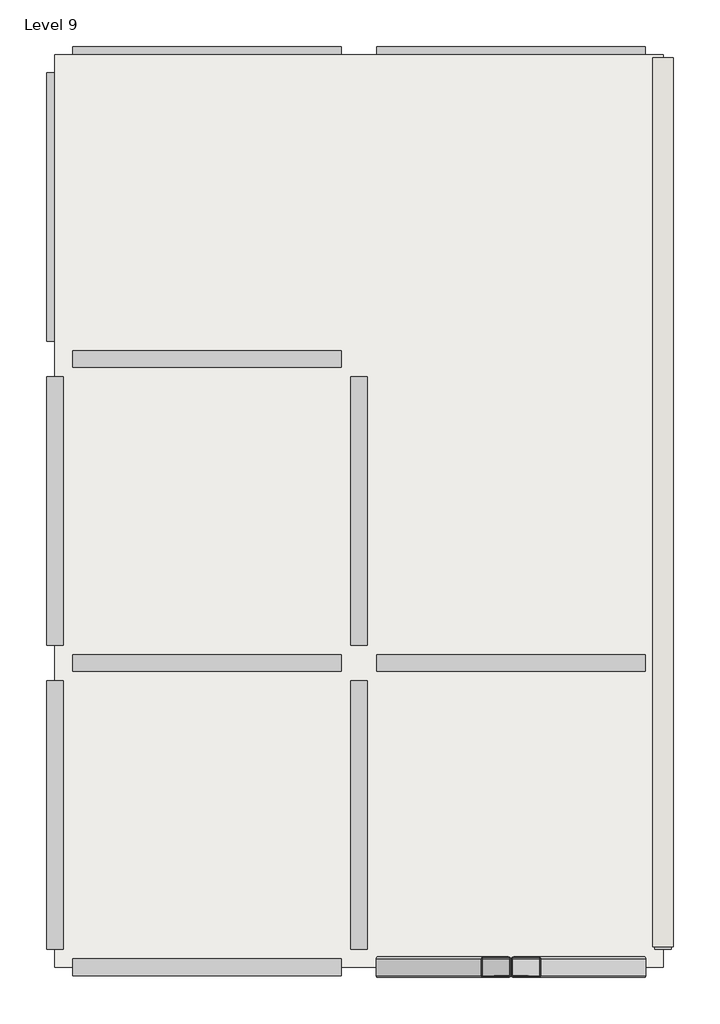
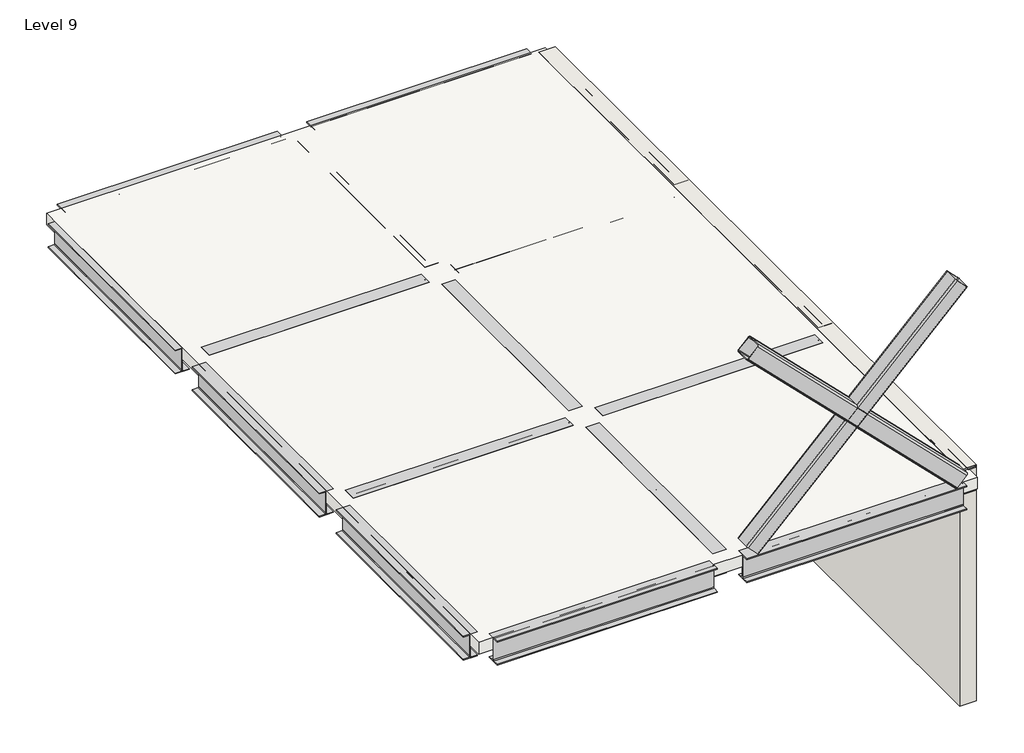
# One storey: 17 beams, 2 members, 1 slab, 1 wall.
"""IFC4 building model written with IfcOpenShell, lengths in millimetres."""

from ifc_helpers import new_model, si_unit, frame, origin, place, context, project, spatial, polyline, outline, extrude, transform, mapped, element, save
from components import ub_universal_beams_ub305x165x40_60ab2ee1, m_hss_square_hss203_2x203_2x9_5_07d005dd

model = new_model("IFC4")

# Units and contexts
model_context = context("Model", 3, world=origin())
ifc_project = project(units=[si_unit("LENGTHUNIT", "METRE", prefix="MILLI")], contexts=[model_context])

# Site, building, storey
site = spatial("IfcSite", under=ifc_project)
building = spatial("IfcBuilding", under=site)
storey = spatial("IfcBuildingStorey", under=building, Name="Level 9", Elevation=24000.0)

# Beams
placement = place(None, origin())
ub_universal_beams_ub305x165x40_shape = ub_universal_beams_ub305x165x40_60ab2ee1(model_context)
element("IfcBeam", 1, ObjectType="UB-Universal Beams : UB305x165x40", at=placement, inside=storey, context=model_context, shape_type="MappedRepresentation", body=[
    mapped(ub_universal_beams_ub305x165x40_shape, transform((18435.1404262, -6314.7314166, 23848.3), x_axis=(-1.0, 0.0, 0.0), y_axis=(0.0, -1.0, 0.0), z_axis=(0.0, 0.0, 1.0))),
])
element("IfcBeam", 2, ObjectType="UB-Universal Beams : UB305x165x40", at=placement, inside=storey, context=model_context, shape_type="MappedRepresentation", body=[
    mapped(ub_universal_beams_ub305x165x40_shape, transform((15435.1404262, -6314.7314166, 23848.3), x_axis=(-1.0, 0.0, 0.0), y_axis=(0.0, -1.0, 0.0), z_axis=(0.0, 0.0, 1.0))),
])
element("IfcBeam", 3, ObjectType="UB-Universal Beams : UB305x165x40", at=placement, inside=storey, context=model_context, shape_type="MappedRepresentation", body=[
    mapped(ub_universal_beams_ub305x165x40_shape, transform((13935.1404262, -4814.7314166, 23848.3), x_axis=(0.0, 1.0, 0.0), y_axis=(-1.0, 0.0, 0.0), z_axis=(0.0, 0.0, 1.0))),
])
element("IfcBeam", 4, ObjectType="UB-Universal Beams : UB305x165x40", at=placement, inside=storey, context=model_context, shape_type="MappedRepresentation", body=[
    mapped(ub_universal_beams_ub305x165x40_shape, transform((13935.1404262, -1814.7314166, 23848.3), x_axis=(0.0, 1.0, 0.0), y_axis=(-1.0, 0.0, 0.0), z_axis=(0.0, 0.0, 1.0))),
])
element("IfcBeam", 5, ObjectType="UB-Universal Beams : UB305x165x40", at=placement, inside=storey, context=model_context, shape_type="MappedRepresentation", body=[
    mapped(ub_universal_beams_ub305x165x40_shape, transform((13935.1404262, 1185.2685834, 23848.3), x_axis=(0.0, 1.0, 0.0), y_axis=(-1.0, 0.0, 0.0), z_axis=(0.0, 0.0, 1.0))),
])
element("IfcBeam", 6, ObjectType="UB-Universal Beams : UB305x165x40", at=placement, inside=storey, context=model_context, shape_type="MappedRepresentation", body=[
    mapped(ub_universal_beams_ub305x165x40_shape, transform((18435.1404262, -3314.7314166, 23848.3), x_axis=(-1.0, 0.0, 0.0), y_axis=(0.0, -1.0, 0.0), z_axis=(0.0, 0.0, 1.0))),
])
element("IfcBeam", 7, ObjectType="UB-Universal Beams : UB305x165x40", at=placement, inside=storey, context=model_context, shape_type="MappedRepresentation", body=[
    mapped(ub_universal_beams_ub305x165x40_shape, transform((15435.1404262, -3314.7314166, 23848.3), x_axis=(-1.0, 0.0, 0.0), y_axis=(0.0, -1.0, 0.0), z_axis=(0.0, 0.0, 1.0))),
])
element("IfcBeam", 8, ObjectType="UB-Universal Beams : UB305x165x40", at=placement, inside=storey, context=model_context, shape_type="MappedRepresentation", body=[
    mapped(ub_universal_beams_ub305x165x40_shape, transform((18435.1404262, -314.7314166, 23848.3), x_axis=(-1.0, 0.0, 0.0), y_axis=(0.0, -1.0, 0.0), z_axis=(0.0, 0.0, 1.0))),
])
element("IfcBeam", 9, ObjectType="UB-Universal Beams : UB305x165x40", at=placement, inside=storey, context=model_context, shape_type="MappedRepresentation", body=[
    mapped(ub_universal_beams_ub305x165x40_shape, transform((15435.1404262, -314.7314166, 23848.3), x_axis=(-1.0, 0.0, 0.0), y_axis=(0.0, -1.0, 0.0), z_axis=(0.0, 0.0, 1.0))),
])
element("IfcBeam", 10, ObjectType="UB-Universal Beams : UB305x165x40", at=placement, inside=storey, context=model_context, shape_type="MappedRepresentation", body=[
    mapped(ub_universal_beams_ub305x165x40_shape, transform((18435.1404262, 2685.2685834, 23848.3), x_axis=(-1.0, 0.0, 0.0), y_axis=(0.0, -1.0, 0.0), z_axis=(0.0, 0.0, 1.0))),
])
element("IfcBeam", 11, ObjectType="UB-Universal Beams : UB305x165x40", at=placement, inside=storey, context=model_context, shape_type="MappedRepresentation", body=[
    mapped(ub_universal_beams_ub305x165x40_shape, transform((15435.1404262, 2685.2685834, 23848.3), x_axis=(-1.0, 0.0, 0.0), y_axis=(0.0, -1.0, 0.0), z_axis=(0.0, 0.0, 1.0))),
])
element("IfcBeam", 12, ObjectType="UB-Universal Beams : UB305x165x40", at=placement, inside=storey, context=model_context, shape_type="MappedRepresentation", body=[
    mapped(ub_universal_beams_ub305x165x40_shape, transform((16935.1404262, -4814.7314166, 23848.3), x_axis=(0.0, 1.0, 0.0), y_axis=(-1.0, 0.0, 0.0), z_axis=(0.0, 0.0, 1.0))),
])
element("IfcBeam", 13, ObjectType="UB-Universal Beams : UB305x165x40", at=placement, inside=storey, context=model_context, shape_type="MappedRepresentation", body=[
    mapped(ub_universal_beams_ub305x165x40_shape, transform((16935.1404262, -1814.7314166, 23848.3), x_axis=(0.0, 1.0, 0.0), y_axis=(-1.0, 0.0, 0.0), z_axis=(0.0, 0.0, 1.0))),
])
element("IfcBeam", 14, ObjectType="UB-Universal Beams : UB305x165x40", at=placement, inside=storey, context=model_context, shape_type="MappedRepresentation", body=[
    mapped(ub_universal_beams_ub305x165x40_shape, transform((16935.1404262, 1185.2685834, 23848.3), x_axis=(0.0, 1.0, 0.0), y_axis=(-1.0, 0.0, 0.0), z_axis=(0.0, 0.0, 1.0))),
])
element("IfcBeam", 15, ObjectType="UB-Universal Beams : UB305x165x40", at=placement, inside=storey, context=model_context, shape_type="MappedRepresentation", body=[
    mapped(ub_universal_beams_ub305x165x40_shape, transform((19935.1404262, -1814.7314166, 23848.3), x_axis=(0.0, 1.0, 0.0), y_axis=(-1.0, 0.0, 0.0), z_axis=(0.0, 0.0, 1.0))),
])
element("IfcBeam", 16, ObjectType="UB-Universal Beams : UB305x165x40", at=placement, inside=storey, context=model_context, shape_type="MappedRepresentation", body=[
    mapped(ub_universal_beams_ub305x165x40_shape, transform((19935.1404262, 1185.2685834, 23848.3), x_axis=(0.0, 1.0, 0.0), y_axis=(-1.0, 0.0, 0.0), z_axis=(0.0, 0.0, 1.0))),
])
element("IfcBeam", 17, ObjectType="UB-Universal Beams : beam", at=placement, inside=storey, context=model_context, shape_type="MappedRepresentation", body=[
    mapped(ub_universal_beams_ub305x165x40_shape, transform((19935.1404262, -4814.7314166, 23848.3), x_axis=(0.0, 1.0, 0.0), y_axis=(-1.0, 0.0, 0.0), z_axis=(0.0, 0.0, 1.0))),
])

# Members
m_hss_square_hss203_2x203_2x9_5_shape = m_hss_square_hss203_2x203_2x9_5_07d005dd(model_context)
element("IfcMember", 18, ObjectType="M_HSS Square : HSS203.2X203.2X9.5", at=placement, inside=storey, context=model_context, shape_type="MappedRepresentation", body=[
    mapped(m_hss_square_hss203_2x203_2x9_5_shape, transform((18435.1404262, -6314.7314166, 25348.3), x_axis=(-0.7071067811865478, 0.0, 0.7071067811865476), y_axis=(0.0, -1.0000000000000002, 0.0), z_axis=(0.7071067811865476, 0.0, 0.7071067811865478))),
])
element("IfcMember", 19, ObjectType="M_HSS Square : HSS203.2X203.2X9.5", at=placement, inside=storey, context=model_context, shape_type="MappedRepresentation", body=[
    mapped(m_hss_square_hss203_2x203_2x9_5_shape, transform((18435.1404262, -6314.7314166, 25348.3), x_axis=(-0.7071067811865478, 0.0, -0.7071067811865475), y_axis=(0.0, -1.0000000000000002, 0.0), z_axis=(-0.7071067811865475, 0.0, 0.7071067811865478))),
])

# Slab
element("IfcSlab", 20, ObjectType="150mm Foundation Slab", at=placement, inside=storey, context=model_context, shape_type="SweptSolid", body=[
    extrude(outline(polyline([(13935.1404262, -6314.7314166), (13935.1404262, 2685.2685834), (19935.1404262, 2685.2685834), (19935.1404262, -6314.7314166), (13935.1404262, -6314.7314166)])), frame((0.0, 0.0, 23850.0), z_axis=(0.0, 0.0, 1.0), x_axis=(1.0, 0.0, 0.0)), (0.0, 0.0, 1.0), 150.0),
])

# Wall
element("IfcWall", 21, ObjectType="Generic - 200mm", at=placement, inside=storey, context=model_context, shape_type="SweptSolid", body=[
    extrude(outline(polyline([(19835.1404262, -6114.7314166), (19835.1404262, 2655.9792615), (20035.1404262, 2655.9792615), (20035.1404262, -6114.7314166), (19835.1404262, -6114.7314166)])), frame((0.0, 0.0, 21000.0), z_axis=(0.0, 0.0, 1.0), x_axis=(1.0, 0.0, 0.0)), (0.0, 0.0, 1.0), 3000.0),
])

save(model, "model.ifc")

# Revit data of these elements
# Type "UB-Universal Beams : UB305x165x40"
#   Section Name Key = "UB305X165X40"
#   Width = 16.5 cm
#   Web Thickness = 0.6 cm
#   Web Fillet = 0.89 cm
#   Warping Constant = 164000.0 cm⁶
#   Torsional Moment of Inertia = 14.70 cm⁴
#   Section Area = 51.3 cm²
#   Plastic Modulus weak axis = 142.0 cm³
#   Plastic Modulus strong axis = 623.0 cm³
#   Nominal Weight = 40.2999 kgf/m
#   Moment of Inertia weak axis = 764.00 cm⁴
#   Moment of Inertia strong axis = 8503.00 cm⁴
#   Height = 30.34 cm
#   Flange Thickness = 1.02 cm
#   Elastic Modulus weak axis = 92.6 cm³
#   Elastic Modulus strong axis = 560.0 cm³
#   Centroid Vertical = 15.17 cm
#   Centroid Horizontal = 8.25 cm
#   Bolt Spacing = 9.0 cm
#   Length [instance default] = 1.5 m
#   Structural Material [instance default] = Metal - Steel 43-275
#   Type Comments = ""
#   Assembly Code = ""
# Type "UB-Universal Beams : beam"
#   Section Name Key = "UB305X165X40"
#   Width = 16.5 cm
#   Web Thickness = 0.6 cm
#   Web Fillet = 0.89 cm
#   Warping Constant = 164000.0 cm⁶
#   Torsional Moment of Inertia = 14.70 cm⁴
#   Section Area = 51.3 cm²
#   Plastic Modulus weak axis = 142.0 cm³
#   Plastic Modulus strong axis = 623.0 cm³
#   Nominal Weight = 40.2999 kgf/m
#   Moment of Inertia weak axis = 764.00 cm⁴
#   Moment of Inertia strong axis = 8503.00 cm⁴
#   Height = 30.34 cm
#   Flange Thickness = 1.02 cm
#   Elastic Modulus weak axis = 92.6 cm³
#   Elastic Modulus strong axis = 560.0 cm³
#   Centroid Vertical = 15.17 cm
#   Centroid Horizontal = 8.25 cm
#   Bolt Spacing = 9.0 cm
#   Length [instance default] = 1.5 m
#   Structural Material [instance default] = Metal - Steel 43-275
#   Type Comments = ""
#   Assembly Code = ""
# Type "M_HSS Square : HSS203.2X203.2X9.5"
#   Section Name Key = "HSS 8X8X3/8"
#   Width = 20.3 cm
#   Wall Nominal Thickness = 0.953 cm
#   Wall Design Thickness = 0.886 cm
#   Torsional Moment of Inertia = 6660.00 cm⁴
#   Torsional Modulus = 10930171.7 cm³
#   Section Area = 67.1 cm²
#   Plastic Modulus weak axis = 482.0 cm³
#   Plastic Modulus strong axis = 482.0 cm³
#   Outer Fillet = 1.906 cm
#   Nominal Weight = 55.9998 kgf/m
#   Moment of Inertia weak axis = 4160.00 cm⁴
#   Moment of Inertia strong axis = 4160.00 cm⁴
#   Length [instance default] = 1.524 m
#   Inner Fillet = 0.953 cm
#   Height = 20.3 cm
#   Elastic Modulus weak axis = 408.0 cm³
#   Elastic Modulus strong axis = 408.0 cm³
#   Centroid Vertical = 10.15 cm
#   Centroid Horizontal = 10.15 cm
#   Structural Material [instance default] = Steel, 45-345
# Type "150mm Foundation Slab"
#   Layers, outside or top first: 0.15 m "Concrete, Cast-in-Place gray" (function 1)
# Type "Generic - 200mm"
#   Layers, outside or top first: 0.2 m no material (function 1)
# Elements 1, 2, 3, 4, 5, 6, 7, 8, 9, 10, 11, 12, 13, 14, 15, 16 (IfcBeam, "UB-Universal Beams : UB305x165x40")
#   Structural Material = Metal - Steel 43-275
#   Phase Created = New Construction
#   Materials on its faces: "Metal - Steel 43-275"
# Element 17 (IfcBeam, "UB-Universal Beams : beam")
#   Structural Material = Metal - Steel 43-275
#   Phase Created = New Construction
#   Materials on its faces: "Metal - Steel 43-275"
# Elements 18, 19 (IfcMember, "M_HSS Square : HSS203.2X203.2X9.5")
#   Comments = ""
#   Structural Material = Metal - Steel 43-275
#   Phase Created = New Construction
#   Materials on its faces: "Metal - Steel 43-275"
# Element 20 (IfcSlab, "150mm Foundation Slab")
#   built-in parameter 1001955 = 3.14159 (stored number, unit not read)
#   Height Offset From Level = 0 m
#   built-in parameter 1001954 = 1
#   Phase Created = New Construction
#   Materials on its faces: "Concrete, Cast-in-Place gray"
# Element 21 (IfcWall, "Generic - 200mm")
#   Comments = ""
#   built-in parameter 1001111 = -3 m
#   Top Offset = 0 m
#   Base Offset = -3 m
#   wall height = 3 m
#   Phase Created = New Construction
#   Base Constraint = Level 9
#   Top Constraint = Level 9
#   Materials on its faces: "Default Wall"
# Materials
#   "Metal - Steel 43-275": class "Metal", colour RGB 247 247 247, transparency 0, Cost = 0
#   "Steel, 45-345": class "Metal", colour RGB 247 247 247, transparency 0, Description = "Steel 345 MPa", Cost = 0
#   "Concrete, Cast-in-Place gray": class "Concrete", colour RGB 192 192 192, transparency 0, Description = "Cast-in-place concrete", Cost = 0
#   "Default Wall": colour RGB 128 128 128, transparency 0, Cost = 0
